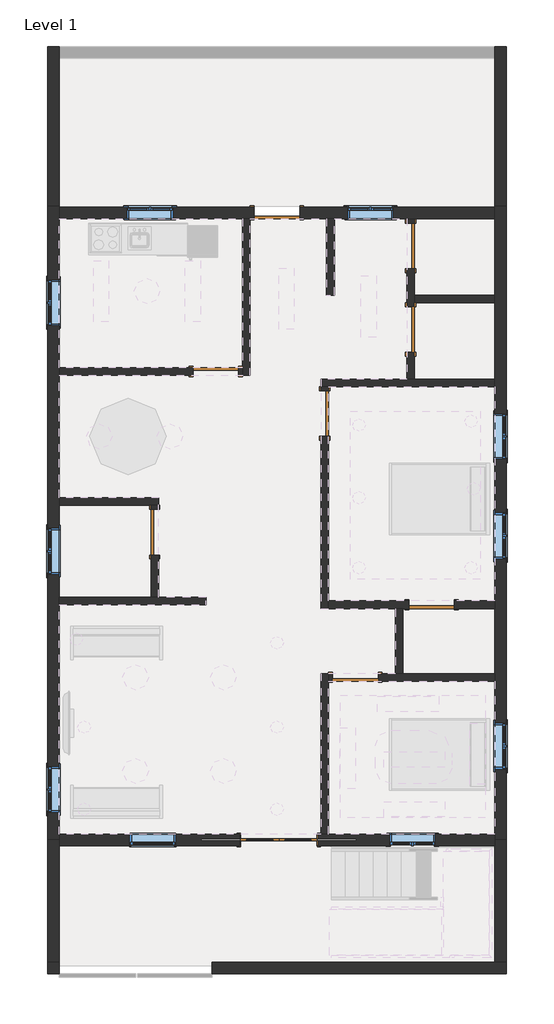
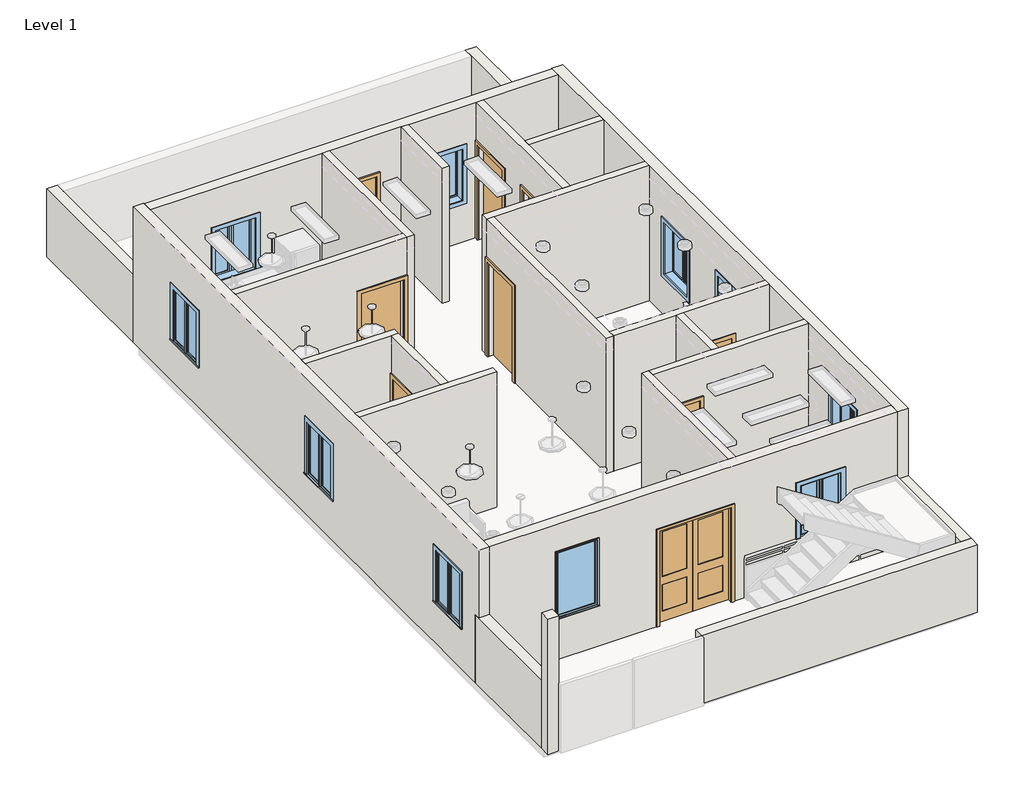
# One storey, part 1 of 2: 24 walls, 10 windows, 9 doors.
"""IFC4 building model written with IfcOpenShell, lengths in millimetres."""

from ifc_helpers import new_model, si_unit, frame, origin, origin_with_axes, place, context, project, spatial, polyline, outline, extrude, faceted_brep, transform, mapped, element, save
from components import door_53d589bd, door_0ca8825f, door_16372e1c, single_flush_single_door_686f89d2, window_419b5846, m_awning_with_trim_0915_x_1220mm_6739fb62

model = new_model("IFC4")

# Units and contexts
model_context = context("Model", 3, world=origin())
ifc_project = project(units=[si_unit("LENGTHUNIT", "METRE", prefix="MILLI")], contexts=[model_context])

# Site, building, storey
site = spatial("IfcSite", under=ifc_project)
building = spatial("IfcBuilding", under=site)
storey = spatial("IfcBuildingStorey", under=building, Name="Level 1", Elevation=0.0)

# Doors
placement = place(None, origin())
door_shape = door_53d589bd(model_context)
element("IfcDoor", 1, ObjectType="Door-Interior-Double-Pocket-2_Panel-Wood : 60\" x 84\"", at=placement, inside=storey, context=model_context, shape_type="MappedRepresentation", body=[
    mapped(door_shape, transform((-5459.0692849, 1586.5206867, 0.0), x_axis=(1.0, 0.0, 0.0), y_axis=(0.0, 1.0, 0.0), z_axis=(0.0, 0.0, 1.0))),
])
door_2_shape = door_0ca8825f(model_context)
element("IfcDoor", 2, ObjectType="Single-Flush : 36\" x 84\"", at=placement, inside=storey, context=model_context, shape_type="MappedRepresentation", body=[
    mapped(door_2_shape, transform((-5497.1692849, 14083.3206867, 0.0), x_axis=(-1.0, 0.0, 0.0), y_axis=(0.0, -1.0, 0.0), z_axis=(0.0, 0.0, 1.0))),
])
door_3_shape = door_16372e1c(model_context)
element("IfcDoor", 3, ObjectType="Single-Flush : 36\" x 84\"", at=placement, inside=storey, context=model_context, shape_type="MappedRepresentation", body=[
    mapped(door_3_shape, transform((-6716.3692849, 10921.0206867, 0.0), x_axis=(1.0, 0.0, 0.0), y_axis=(0.0, 1.0, 0.0), z_axis=(0.0, 0.0, 1.0))),
])
element("IfcDoor", 4, ObjectType="Single-Flush : single door", at=placement, inside=storey, context=model_context, shape_type="MappedRepresentation", body=[
    mapped(door_3_shape, transform((-3935.0692849, 4825.0206867, 0.0), x_axis=(-1.0, 0.0, 0.0), y_axis=(0.0, -1.0, 0.0), z_axis=(0.0, 0.0, 1.0))),
])
element("IfcDoor", 5, ObjectType="Single-Flush : single door", at=placement, inside=storey, context=model_context, shape_type="MappedRepresentation", body=[
    mapped(door_3_shape, transform((-2411.0692849, 6272.8206867, 0.0), x_axis=(-1.0, 0.0, 0.0), y_axis=(0.0, -1.0, 0.0), z_axis=(0.0, 0.0, 1.0))),
])
element("IfcDoor", 6, ObjectType="Single-Flush : single door", at=placement, inside=storey, context=model_context, shape_type="MappedRepresentation", body=[
    mapped(door_3_shape, transform((-7935.5692849, 7720.6206867, 0.0), x_axis=(0.0, 1.0, 0.0), y_axis=(-1.0, 0.0, 0.0), z_axis=(0.0, 0.0, 1.0))),
])
single_flush_single_door_shape = single_flush_single_door_686f89d2(model_context)
element("IfcDoor", 7, ObjectType="Single-Flush : single door", at=placement, inside=storey, context=model_context, shape_type="MappedRepresentation", body=[
    mapped(single_flush_single_door_shape, transform((-4544.6692849, 10082.8206867, 0.0), x_axis=(0.0, 1.0, 0.0), y_axis=(-1.0, 0.0, 0.0), z_axis=(0.0, 0.0, 1.0))),
])
element("IfcDoor", 8, ObjectType="Single-Flush : single door", at=placement, inside=storey, context=model_context, shape_type="MappedRepresentation", body=[
    mapped(single_flush_single_door_shape, transform((-2830.1692849, 13422.9206867, 0.0), x_axis=(0.0, 1.0, 0.0), y_axis=(-1.0, 0.0, 0.0), z_axis=(0.0, 0.0, 1.0))),
])
element("IfcDoor", 9, ObjectType="Single-Flush : single door", at=placement, inside=storey, context=model_context, shape_type="MappedRepresentation", body=[
    mapped(single_flush_single_door_shape, transform((-2830.1692849, 11759.2206867, 0.0), x_axis=(0.0, 1.0, 0.0), y_axis=(-1.0, 0.0, 0.0), z_axis=(0.0, 0.0, 1.0))),
])

# Walls
element("IfcWall", 10, ObjectType="6\"", at=placement, inside=storey, context=model_context, shape_type="Brep", body=[
    faceted_brep([(-4468.4692849, 1700.8206867, 0.0), (-4468.4692849, 4748.8206867, 0.0), (-4468.4692849, 4901.2206867, 0.0), (-4468.4692849, 4901.2206867, 3048.0), (-4468.4692849, 4748.8206867, 3048.0), (-4468.4692849, 1700.8206867, 3048.0), (-4620.8692849, 1700.8206867, 0.0), (-4620.8692849, 1700.8206867, 3048.0), (-4620.8692849, 4901.2206867, 3048.0), (-4620.8692849, 4901.2206867, 0.0)], [[[0, 1, 2, 3, 4, 5]], [[6, 7, 8, 9]], [[2, 1, 0, 6, 9]], [[5, 4, 3, 8, 7]], [[0, 5, 7, 6]], [[3, 2, 9, 8]]]),
])
element("IfcWall", 11, ObjectType="6\"", at=placement, inside=storey, context=model_context, shape_type="Brep", body=[
    faceted_brep([(-4392.2692849, 4901.2206867, 2133.6), (-4392.2692849, 4901.2206867, 0.0), (-4468.4692849, 4901.2206867, 0.0), (-4468.4692849, 4901.2206867, 3048.0), (-3134.9692849, 4901.2206867, 3048.0), (-2982.5692849, 4901.2206867, 3048.0), (-1153.7692849, 4901.2206867, 3048.0), (-1153.7692849, 4901.2206867, 0.0), (-2982.5692849, 4901.2206867, 0.0), (-3134.9692849, 4901.2206867, 0.0), (-3477.8692849, 4901.2206867, 0.0), (-3477.8692849, 4901.2206867, 2133.6), (-4468.4692849, 4748.8206867, 0.0), (-4392.2692849, 4748.8206867, 0.0), (-4392.2692849, 4748.8206867, 2133.6), (-3477.8692849, 4748.8206867, 2133.6), (-3477.8692849, 4748.8206867, 0.0), (-1153.7692849, 4748.8206867, 0.0), (-1153.7692849, 4748.8206867, 3048.0), (-4468.4692849, 4748.8206867, 3048.0)], [[[0, 1, 2, 3, 4, 5, 6, 7, 8, 9, 10, 11]], [[12, 13, 14, 15, 16, 17, 18, 19]], [[2, 1, 13, 12]], [[10, 9, 8, 7, 17, 16]], [[6, 5, 4, 3, 19, 18]], [[7, 6, 18, 17]], [[3, 2, 12, 19]], [[14, 13, 1, 0]], [[15, 14, 0, 11]], [[16, 15, 11, 10]]]),
])
element("IfcWall", 12, ObjectType="6\"", at=placement, inside=storey, context=model_context, shape_type="SweptSolid", body=[
    extrude(outline(polyline([(-2982.5692849, 6196.6206867), (-2982.5692849, 4901.2206867), (-3134.9692849, 4901.2206867), (-3134.9692849, 6196.6206867), (-2982.5692849, 6196.6206867)])), origin_with_axes(), (0.0, 0.0, 1.0), 3048.0),
])
element("IfcWall", 13, ObjectType="6\"", at=placement, inside=storey, context=model_context, shape_type="Brep", body=[
    faceted_brep([(-4468.4692849, 6349.0206867, 3048.0), (-1153.7692849, 6349.0206867, 3048.0), (-1153.7692849, 6349.0206867, 0.0), (-1953.8692849, 6349.0206867, 0.0), (-1953.8692849, 6349.0206867, 2133.6), (-2868.2692849, 6349.0206867, 2133.6), (-2868.2692849, 6349.0206867, 0.0), (-4468.4692849, 6349.0206867, 0.0), (-1153.7692849, 6196.6206867, 3048.0), (-2982.5692849, 6196.6206867, 3048.0), (-3134.9692849, 6196.6206867, 3048.0), (-4468.4692849, 6196.6206867, 3048.0), (-4468.4692849, 6196.6206867, 0.0), (-3134.9692849, 6196.6206867, 0.0), (-2982.5692849, 6196.6206867, 0.0), (-2868.2692849, 6196.6206867, 0.0), (-2868.2692849, 6196.6206867, 2133.6), (-1953.8692849, 6196.6206867, 2133.6), (-1953.8692849, 6196.6206867, 0.0), (-1153.7692849, 6196.6206867, 0.0)], [[[0, 1, 2, 3, 4, 5, 6, 7]], [[8, 9, 10, 11, 12, 13, 14, 15, 16, 17, 18, 19]], [[2, 19, 18, 3]], [[12, 7, 6, 15, 14, 13]], [[1, 0, 11, 10, 9, 8]], [[2, 1, 8, 19]], [[0, 7, 12, 11]], [[16, 5, 4, 17]], [[17, 4, 3, 18]], [[5, 16, 15, 6]]]),
])
element("IfcWall", 14, ObjectType="6\"", at=placement, inside=storey, context=model_context, shape_type="Brep", body=[
    faceted_brep([(-1153.7692849, 10768.6206867, 0.0), (-2753.9692849, 10768.6206867, 0.0), (-2906.3692849, 10768.6206867, 0.0), (-4620.8692849, 10768.6206867, 0.0), (-4620.8692849, 10768.6206867, 3048.0), (-2906.3692849, 10768.6206867, 3048.0), (-2753.9692849, 10768.6206867, 3048.0), (-1153.7692849, 10768.6206867, 3048.0), (-1153.7692849, 10616.2206867, 0.0), (-1153.7692849, 10616.2206867, 3048.0), (-4468.4692849, 10616.2206867, 3048.0), (-4620.8692849, 10616.2206867, 3048.0), (-4620.8692849, 10616.2206867, 0.0), (-4468.4692849, 10616.2206867, 0.0)], [[[0, 1, 2, 3, 4, 5, 6, 7]], [[8, 9, 10, 11, 12, 13]], [[3, 2, 1, 0, 8, 13, 12]], [[7, 6, 5, 4, 11, 10, 9]], [[0, 7, 9, 8]], [[4, 3, 12, 11]]]),
])
element("IfcWall", 15, ObjectType="6\"", at=placement, inside=storey, context=model_context, shape_type="Brep", body=[
    faceted_brep([(-4468.4692849, 10540.0206867, 2133.6), (-4468.4692849, 10540.0206867, 0.0), (-4468.4692849, 10616.2206867, 0.0), (-4468.4692849, 10616.2206867, 3048.0), (-4468.4692849, 6349.0206867, 3048.0), (-4468.4692849, 6196.6206867, 3048.0), (-4468.4692849, 6196.6206867, 0.0), (-4468.4692849, 6349.0206867, 0.0), (-4468.4692849, 9625.6206867, 0.0), (-4468.4692849, 9625.6206867, 2133.6), (-4620.8692849, 10616.2206867, 0.0), (-4620.8692849, 10540.0206867, 0.0), (-4620.8692849, 10540.0206867, 2133.6), (-4620.8692849, 9625.6206867, 2133.6), (-4620.8692849, 9625.6206867, 0.0), (-4620.8692849, 6196.6206867, 0.0), (-4620.8692849, 6196.6206867, 3048.0), (-4620.8692849, 10616.2206867, 3048.0)], [[[0, 1, 2, 3, 4, 5, 6, 7, 8, 9]], [[10, 11, 12, 13, 14, 15, 16, 17]], [[2, 1, 11, 10]], [[8, 7, 6, 15, 14]], [[5, 4, 3, 17, 16]], [[3, 2, 10, 17]], [[6, 5, 16, 15]], [[12, 11, 1, 0]], [[13, 12, 0, 9]], [[14, 13, 9, 8]]]),
])
element("IfcWall", 16, ObjectType="6\"", at=placement, inside=storey, context=model_context, shape_type="SweptSolid", body=[
    extrude(outline(polyline([(-2753.9692849, 12445.0206867), (-1153.7692849, 12445.0206867), (-1153.7692849, 12292.6206867), (-2753.9692849, 12292.6206867), (-2753.9692849, 12445.0206867)])), origin_with_axes(), (0.0, 0.0, 1.0), 3048.0),
])
element("IfcWall", 17, ObjectType="6\"", at=placement, inside=storey, context=model_context, shape_type="Brep", body=[
    faceted_brep([(-2753.9692849, 12216.4206867, 2133.6), (-2753.9692849, 12216.4206867, 0.0), (-2753.9692849, 12292.6206867, 0.0), (-2753.9692849, 12445.0206867, 0.0), (-2753.9692849, 12965.7206867, 0.0), (-2753.9692849, 12965.7206867, 2133.6), (-2753.9692849, 13880.1206867, 2133.6), (-2753.9692849, 13880.1206867, 0.0), (-2753.9692849, 13969.0206867, 0.0), (-2753.9692849, 13969.0206867, 3048.0), (-2753.9692849, 12445.0206867, 3048.0), (-2753.9692849, 12292.6206867, 3048.0), (-2753.9692849, 10768.6206867, 3048.0), (-2753.9692849, 10768.6206867, 0.0), (-2753.9692849, 11302.0206867, 0.0), (-2753.9692849, 11302.0206867, 2133.6), (-2906.3692849, 12965.7206867, 0.0), (-2906.3692849, 12216.4206867, 0.0), (-2906.3692849, 12216.4206867, 2133.6), (-2906.3692849, 11302.0206867, 2133.6), (-2906.3692849, 11302.0206867, 0.0), (-2906.3692849, 10768.6206867, 0.0), (-2906.3692849, 10768.6206867, 3048.0), (-2906.3692849, 13969.0206867, 3048.0), (-2906.3692849, 13969.0206867, 0.0), (-2906.3692849, 13880.1206867, 0.0), (-2906.3692849, 13880.1206867, 2133.6), (-2906.3692849, 12965.7206867, 2133.6)], [[[0, 1, 2, 3, 4, 5, 6, 7, 8, 9, 10, 11, 12, 13, 14, 15]], [[16, 17, 18, 19, 20, 21, 22, 23, 24, 25, 26, 27]], [[8, 7, 25, 24]], [[14, 13, 21, 20]], [[4, 3, 2, 1, 17, 16]], [[12, 11, 10, 9, 23, 22]], [[13, 12, 22, 21]], [[9, 8, 24, 23]], [[26, 25, 7, 6]], [[27, 26, 6, 5]], [[16, 27, 5, 4]], [[18, 17, 1, 0]], [[19, 18, 0, 15]], [[20, 19, 15, 14]]]),
])
element("IfcWall", 18, ObjectType="6\"", at=placement, inside=storey, context=model_context, shape_type="Brep", body=[
    faceted_brep([(-6182.9692849, 13969.0206867, 0.0), (-6182.9692849, 10997.2206867, 0.0), (-6182.9692849, 10844.8206867, 0.0), (-6182.9692849, 10844.8206867, 3048.0), (-6182.9692849, 10997.2206867, 3048.0), (-6182.9692849, 13969.0206867, 3048.0), (-6030.5692849, 13969.0206867, 0.0), (-6030.5692849, 13969.0206867, 3048.0), (-6030.5692849, 10844.8206867, 3048.0), (-6030.5692849, 10844.8206867, 0.0)], [[[0, 1, 2, 3, 4, 5]], [[6, 7, 8, 9]], [[2, 1, 0, 6, 9]], [[5, 4, 3, 8, 7]], [[0, 5, 7, 6]], [[3, 2, 9, 8]]]),
])
element("IfcWall", 19, ObjectType="6\"", at=placement, inside=storey, context=model_context, shape_type="Brep", body=[
    faceted_brep([(-9840.5692849, 8254.0206867, 0.0), (-8011.7692849, 8254.0206867, 0.0), (-7859.3692849, 8254.0206867, 0.0), (-7859.3692849, 8254.0206867, 3048.0), (-8011.7692849, 8254.0206867, 3048.0), (-9840.5692849, 8254.0206867, 3048.0), (-9840.5692849, 8406.4206867, 0.0), (-9840.5692849, 8406.4206867, 3048.0), (-7859.3692849, 8406.4206867, 3048.0), (-7859.3692849, 8406.4206867, 0.0)], [[[0, 1, 2, 3, 4, 5]], [[6, 7, 8, 9]], [[2, 1, 0, 6, 9]], [[5, 4, 3, 8, 7]], [[0, 5, 7, 6]], [[3, 2, 9, 8]]]),
])
element("IfcWall", 20, ObjectType="6\"", at=placement, inside=storey, context=model_context, shape_type="SweptSolid", body=[
    extrude(outline(polyline([(8254.0206867, 0.0), (8177.8206867, 0.0), (8177.8206867, 2133.6), (7263.4206867, 2133.6), (7263.4206867, 0.0), (6425.2206867, 0.0), (6425.2206867, 3048.0), (8254.0206867, 3048.0), (8254.0206867, 0.0)])), frame((-8011.7692849, 0.0, 0.0), z_axis=(1.0, 0.0, 0.0), x_axis=(0.0, 1.0, 0.0)), (0.0, 0.0, 1.0), 152.4),
])
element("IfcWall", 21, ObjectType="6\"", at=placement, inside=storey, context=model_context, shape_type="Brep", body=[
    faceted_brep([(-6906.8692849, 6425.2206867, 0.0), (-7859.3692849, 6425.2206867, 0.0), (-8011.7692849, 6425.2206867, 0.0), (-9840.5692849, 6425.2206867, 0.0), (-9840.5692849, 6425.2206867, 3048.0), (-8011.7692849, 6425.2206867, 3048.0), (-7859.3692849, 6425.2206867, 3048.0), (-6906.8692849, 6425.2206867, 3048.0), (-6906.8692849, 6272.8206867, 0.0), (-6906.8692849, 6272.8206867, 3048.0), (-9840.5692849, 6272.8206867, 3048.0), (-9840.5692849, 6272.8206867, 0.0)], [[[0, 1, 2, 3, 4, 5, 6, 7]], [[8, 9, 10, 11]], [[3, 2, 1, 0, 8, 11]], [[7, 6, 5, 4, 10, 9]], [[0, 7, 9, 8]], [[4, 3, 11, 10]]]),
])
element("IfcWall", 22, ObjectType="6\"", at=placement, inside=storey, context=model_context, shape_type="SweptSolid", body=[
    extrude(outline(polyline([(2133.6, -6259.1692849), (0.0, -6259.1692849), (0.0, -6182.9692849), (3048.0, -6182.9692849), (3048.0, -9840.5692849), (0.0, -9840.5692849), (0.0, -7173.5692849), (2133.6, -7173.5692849), (2133.6, -6259.1692849)])), frame((0.0, 10844.8206867, 0.0), z_axis=(0.0, 1.0, 0.0), x_axis=(0.0, 0.0, 1.0)), (0.0, 0.0, 1.0), 152.4),
])
element("IfcWall", 23, ObjectType="6\"", at=placement, inside=storey, context=model_context, shape_type="SweptSolid", body=[
    extrude(outline(polyline([(-4506.5692849, 12445.0206867), (-4506.5692849, 13969.0206867), (-4354.1692849, 13969.0206867), (-4354.1692849, 12445.0206867), (-4506.5692849, 12445.0206867)])), origin_with_axes(), (0.0, 0.0, 1.0), 3048.0),
])
element("IfcWall", 24, ObjectType="9\"", at=placement, inside=storey, context=model_context, shape_type="Brep", body=[
    faceted_brep([(-9840.5692849, -851.8793133, 0.0), (-9840.5692849, 1472.2206867, 0.0), (-9840.5692849, 1586.5206867, 0.0), (-9840.5692849, 1586.5206867, 1524.0), (-9840.5692849, 1472.2206867, 1524.0), (-9840.5692849, -851.8793133, 1524.0), (-10069.1692849, -851.8793133, 0.0), (-10069.1692849, -851.8793133, 1524.0), (-10069.1692849, 1472.2206867, 1524.0), (-10069.1692849, 1586.5206867, 1524.0), (-10069.1692849, 1586.5206867, 0.0)], [[[0, 1, 2, 3, 4, 5]], [[6, 7, 8, 9, 10]], [[2, 1, 0, 6, 10]], [[3, 2, 10, 9]], [[5, 4, 3, 9, 8, 7]], [[0, 5, 7, 6]]]),
])
element("IfcWall", 25, ObjectType="9\"", at=placement, inside=storey, context=model_context, shape_type="Brep", body=[
    faceted_brep([(-1153.7692849, 17398.0206867, 0.0), (-1153.7692849, 17169.4206867, 0.0), (-1153.7692849, 14210.3206867, 0.0), (-1153.7692849, 14210.3206867, 1524.0), (-1153.7692849, 17169.4206867, 1524.0), (-1153.7692849, 17398.0206867, 1524.0), (-925.1692849, 17398.0206867, 0.0), (-925.1692849, 17398.0206867, 1524.0), (-925.1692849, 14210.3206867, 1524.0), (-925.1692849, 14210.3206867, 0.0)], [[[0, 1, 2, 3, 4, 5]], [[6, 7, 8, 9]], [[2, 1, 0, 6, 9]], [[3, 2, 9, 8]], [[5, 4, 3, 8, 7]], [[0, 5, 7, 6]]]),
])
element("IfcWall", 26, ObjectType="9\"", at=placement, inside=storey, context=model_context, shape_type="Brep", body=[
    faceted_brep([(-9840.5692849, 1700.8206867, 3048.0), (-4620.8692849, 1700.8206867, 3048.0), (-4468.4692849, 1700.8206867, 3048.0), (-1153.7692849, 1700.8206867, 3048.0), (-1153.7692849, 1700.8206867, 0.0), (-4468.4692849, 1700.8206867, 0.0), (-4620.8692849, 1700.8206867, 0.0), (-4671.6692849, 1700.8206867, 0.0), (-4671.6692849, 1700.8206867, 2159.0), (-6246.4692849, 1700.8206867, 2159.0), (-6246.4692849, 1700.8206867, 0.0), (-9840.5692849, 1700.8206867, 0.0), (-3249.2692849, 1700.8206867, 2133.6), (-3249.2692849, 1700.8206867, 914.4), (-2334.8692849, 1700.8206867, 914.4), (-2334.8692849, 1700.8206867, 2133.6), (-8431.1692849, 1700.8206867, 2439.0), (-8431.1692849, 1700.8206867, 915.0), (-7516.1692849, 1700.8206867, 915.0), (-7516.1692849, 1700.8206867, 2439.0), (-1153.7692849, 1472.2206867, 3048.0), (-9840.5692849, 1472.2206867, 3048.0), (-9840.5692849, 1472.2206867, 1524.0), (-9840.5692849, 1472.2206867, 0.0), (-6246.4692849, 1472.2206867, 0.0), (-6246.4692849, 1472.2206867, 2159.0), (-4671.6692849, 1472.2206867, 2159.0), (-4671.6692849, 1472.2206867, 0.0), (-1153.7692849, 1472.2206867, 0.0), (-1153.7692849, 1472.2206867, 1524.0), (-3249.2692849, 1472.2206867, 2133.6), (-2334.8692849, 1472.2206867, 2133.6), (-2334.8692849, 1472.2206867, 914.4), (-3249.2692849, 1472.2206867, 914.4), (-8431.1692849, 1472.2206867, 2439.0), (-7516.1692849, 1472.2206867, 2439.0), (-7516.1692849, 1472.2206867, 915.0), (-8431.1692849, 1472.2206867, 915.0), (-1153.7692849, 1586.5206867, 0.0), (-4671.6692849, 1565.8831867, 0.0), (-3909.6692849, 1565.8831867, 0.0), (-3909.6692849, 1607.1581867, 0.0), (-4671.6692849, 1607.1581867, 0.0), (-9840.5692849, 1586.5206867, 0.0), (-6246.4692849, 1607.1581867, 0.0), (-7008.4692849, 1607.1581867, 0.0), (-7008.4692849, 1565.8831867, 0.0), (-6246.4692849, 1565.8831867, 0.0), (-3909.6692849, 1607.1581867, 2159.0), (-3909.6692849, 1565.8831867, 2159.0), (-4671.6692849, 1565.8831867, 2159.0), (-6246.4692849, 1565.8831867, 2159.0), (-7008.4692849, 1565.8831867, 2159.0), (-7008.4692849, 1607.1581867, 2159.0), (-6246.4692849, 1607.1581867, 2159.0), (-4671.6692849, 1607.1581867, 2159.0)], [[[0, 1, 2, 3, 4, 5, 6, 7, 8, 9, 10, 11], [12, 13, 14, 15], [16, 17, 18, 19]], [[20, 21, 22, 23, 24, 25, 26, 27, 28, 29], [30, 31, 32, 33], [34, 35, 36, 37]], [[4, 38, 28, 27, 39, 40, 41, 42, 7, 6, 5]], [[23, 43, 11, 10, 44, 45, 46, 47, 24]], [[3, 2, 1, 0, 21, 20]], [[13, 12, 30, 33]], [[14, 13, 33, 32]], [[15, 14, 32, 31]], [[12, 15, 31, 30]], [[48, 49, 50, 26, 25, 51, 52, 53, 54, 9, 8, 55]], [[48, 55, 42, 41]], [[55, 8, 7, 42]], [[9, 54, 44, 10]], [[54, 53, 45, 44]], [[53, 52, 46, 45]], [[52, 51, 47, 46]], [[51, 25, 24, 47]], [[26, 50, 39, 27]], [[50, 49, 40, 39]], [[49, 48, 41, 40]], [[11, 43, 23, 22, 21, 0]], [[28, 38, 4, 3, 20, 29]], [[17, 16, 34, 37]], [[18, 17, 37, 36]], [[19, 18, 36, 35]], [[16, 19, 35, 34]]]),
])
element("IfcWall", 27, ObjectType="9\"", at=placement, inside=storey, context=model_context, shape_type="Brep", body=[
    faceted_brep([(-5954.3692849, 14197.6206867, 2133.6), (-5954.3692849, 14197.6206867, 0.0), (-9840.5692849, 14197.6206867, 0.0), (-9840.5692849, 14197.6206867, 3048.0), (-1153.7692849, 14197.6206867, 3048.0), (-1153.7692849, 14197.6206867, 0.0), (-5039.9692849, 14197.6206867, 0.0), (-5039.9692849, 14197.6206867, 2133.6), (-7573.6192849, 14197.6206867, 2133.6), (-8488.0192849, 14197.6206867, 2133.6), (-8488.0192849, 14197.6206867, 914.4), (-7573.6192849, 14197.6206867, 914.4), (-3173.0692849, 14197.6206867, 2133.6), (-4087.4692849, 14197.6206867, 2133.6), (-4087.4692849, 14197.6206867, 914.4), (-3173.0692849, 14197.6206867, 914.4), (-9840.5692849, 13969.0206867, 0.0), (-6182.9692849, 13969.0206867, 0.0), (-6030.5692849, 13969.0206867, 0.0), (-5954.3692849, 13969.0206867, 0.0), (-5954.3692849, 13969.0206867, 2133.6), (-5039.9692849, 13969.0206867, 2133.6), (-5039.9692849, 13969.0206867, 0.0), (-4506.5692849, 13969.0206867, 0.0), (-4354.1692849, 13969.0206867, 0.0), (-2906.3692849, 13969.0206867, 0.0), (-2753.9692849, 13969.0206867, 0.0), (-1153.7692849, 13969.0206867, 0.0), (-1153.7692849, 13969.0206867, 3048.0), (-2753.9692849, 13969.0206867, 3048.0), (-2906.3692849, 13969.0206867, 3048.0), (-4354.1692849, 13969.0206867, 3048.0), (-4506.5692849, 13969.0206867, 3048.0), (-6030.5692849, 13969.0206867, 3048.0), (-6182.9692849, 13969.0206867, 3048.0), (-9840.5692849, 13969.0206867, 3048.0), (-7573.6192849, 13969.0206867, 2133.6), (-7573.6192849, 13969.0206867, 914.4), (-8488.0192849, 13969.0206867, 914.4), (-8488.0192849, 13969.0206867, 2133.6), (-3173.0692849, 13969.0206867, 2133.6), (-3173.0692849, 13969.0206867, 914.4), (-4087.4692849, 13969.0206867, 914.4), (-4087.4692849, 13969.0206867, 2133.6)], [[[0, 1, 2, 3, 4, 5, 6, 7], [8, 9, 10, 11], [12, 13, 14, 15]], [[16, 17, 18, 19, 20, 21, 22, 23, 24, 25, 26, 27, 28, 29, 30, 31, 32, 33, 34, 35], [36, 37, 38, 39], [40, 41, 42, 43]], [[6, 5, 27, 26, 25, 24, 23, 22]], [[2, 1, 19, 18, 17, 16]], [[4, 3, 35, 34, 33, 32, 31, 30, 29, 28]], [[3, 2, 16, 35]], [[5, 4, 28, 27]], [[37, 36, 8, 11]], [[38, 37, 11, 10]], [[39, 38, 10, 9]], [[36, 39, 9, 8]], [[41, 40, 12, 15]], [[42, 41, 15, 14]], [[43, 42, 14, 13]], [[40, 43, 13, 12]], [[20, 19, 1, 0]], [[21, 20, 0, 7]], [[22, 21, 7, 6]]]),
])
element("IfcWall", 28, ObjectType="9\"", at=placement, inside=storey, context=model_context, shape_type="Brep", body=[
    faceted_brep([(-9840.5692849, 1586.5206867, 0.0), (-9840.5692849, 1700.8206867, 0.0), (-9840.5692849, 6272.8206867, 0.0), (-9840.5692849, 6425.2206867, 0.0), (-9840.5692849, 8254.0206867, 0.0), (-9840.5692849, 8406.4206867, 0.0), (-9840.5692849, 10844.8206867, 0.0), (-9840.5692849, 10997.2206867, 0.0), (-9840.5692849, 13969.0206867, 0.0), (-9840.5692849, 14197.6206867, 0.0), (-9840.5692849, 14210.3206867, 0.0), (-9840.5692849, 14210.3206867, 1524.0), (-9840.5692849, 14210.3206867, 3048.0), (-9840.5692849, 14197.6206867, 3048.0), (-9840.5692849, 13969.0206867, 3048.0), (-9840.5692849, 10997.2206867, 3048.0), (-9840.5692849, 10844.8206867, 3048.0), (-9840.5692849, 8406.4206867, 3048.0), (-9840.5692849, 8254.0206867, 3048.0), (-9840.5692849, 6425.2206867, 3048.0), (-9840.5692849, 6272.8206867, 3048.0), (-9840.5692849, 1700.8206867, 3048.0), (-9840.5692849, 1472.2206867, 3048.0), (-9840.5692849, 1472.2206867, 1524.0), (-9840.5692849, 1586.5206867, 1524.0), (-9840.5692849, 3047.0206867, 2133.6), (-9840.5692849, 3047.0206867, 914.4), (-9840.5692849, 2132.6206867, 914.4), (-9840.5692849, 2132.6206867, 2133.6), (-9840.5692849, 7796.8206867, 2133.6), (-9840.5692849, 7796.8206867, 914.4), (-9840.5692849, 6882.4206867, 914.4), (-9840.5692849, 6882.4206867, 2133.6), (-9840.5692849, 12749.8206867, 2133.6), (-9840.5692849, 12749.8206867, 914.4), (-9840.5692849, 11835.4206867, 914.4), (-9840.5692849, 11835.4206867, 2133.6), (-10069.1692849, 1586.5206867, 0.0), (-10069.1692849, 1586.5206867, 1524.0), (-10069.1692849, 1472.2206867, 1524.0), (-10069.1692849, 1472.2206867, 3048.0), (-10069.1692849, 14210.3206867, 3048.0), (-10069.1692849, 14210.3206867, 1524.0), (-10069.1692849, 14210.3206867, 0.0), (-10069.1692849, 3047.0206867, 2133.6), (-10069.1692849, 2132.6206867, 2133.6), (-10069.1692849, 2132.6206867, 914.4), (-10069.1692849, 3047.0206867, 914.4), (-10069.1692849, 7796.8206867, 2133.6), (-10069.1692849, 6882.4206867, 2133.6), (-10069.1692849, 6882.4206867, 914.4), (-10069.1692849, 7796.8206867, 914.4), (-10069.1692849, 12749.8206867, 2133.6), (-10069.1692849, 11835.4206867, 2133.6), (-10069.1692849, 11835.4206867, 914.4), (-10069.1692849, 12749.8206867, 914.4)], [[[0, 1, 2, 3, 4, 5, 6, 7, 8, 9, 10, 11, 12, 13, 14, 15, 16, 17, 18, 19, 20, 21, 22, 23, 24], [25, 26, 27, 28], [29, 30, 31, 32], [33, 34, 35, 36]], [[37, 38, 39, 40, 41, 42, 43], [44, 45, 46, 47], [48, 49, 50, 51], [52, 53, 54, 55]], [[10, 9, 8, 7, 6, 5, 4, 3, 2, 1, 0, 37, 43]], [[12, 11, 10, 43, 42, 41]], [[22, 21, 20, 19, 18, 17, 16, 15, 14, 13, 12, 41, 40]], [[25, 28, 45, 44]], [[28, 27, 46, 45]], [[27, 26, 47, 46]], [[26, 25, 44, 47]], [[29, 32, 49, 48]], [[32, 31, 50, 49]], [[31, 30, 51, 50]], [[30, 29, 48, 51]], [[33, 36, 53, 52]], [[36, 35, 54, 53]], [[35, 34, 55, 54]], [[34, 33, 52, 55]], [[0, 24, 38, 37]], [[23, 39, 38, 24]], [[23, 22, 40, 39]]]),
])
element("IfcWall", 29, ObjectType="9\"", at=placement, inside=storey, context=model_context, shape_type="Brep", body=[
    faceted_brep([(-1153.7692849, 1586.5206867, 0.0), (-1153.7692849, 1472.2206867, 0.0), (-1153.7692849, -851.8793133, 0.0), (-1153.7692849, -851.8793133, 1524.0), (-1153.7692849, 1472.2206867, 1524.0), (-1153.7692849, 1586.5206867, 1524.0), (-925.1692849, 1586.5206867, 0.0), (-925.1692849, 1586.5206867, 1524.0), (-925.1692849, 1472.2206867, 1524.0), (-925.1692849, -851.8793133, 1524.0), (-925.1692849, -851.8793133, 0.0)], [[[0, 1, 2, 3, 4, 5]], [[6, 7, 8, 9, 10]], [[2, 1, 0, 6, 10]], [[5, 4, 3, 9, 8, 7]], [[0, 5, 7, 6]], [[3, 2, 10, 9]]]),
])
element("IfcWall", 30, ObjectType="9\"", at=placement, inside=storey, context=model_context, shape_type="Brep", body=[
    faceted_brep([(-9840.5692849, 14210.3206867, 0.0), (-9840.5692849, 17169.4206867, 0.0), (-9840.5692849, 17398.0206867, 0.0), (-9840.5692849, 17398.0206867, 1524.0), (-9840.5692849, 17169.4206867, 1524.0), (-9840.5692849, 14210.3206867, 1524.0), (-10069.1692849, 14210.3206867, 0.0), (-10069.1692849, 14210.3206867, 1524.0), (-10069.1692849, 17398.0206867, 1524.0), (-10069.1692849, 17398.0206867, 0.0)], [[[0, 1, 2, 3, 4, 5]], [[6, 7, 8, 9]], [[2, 1, 0, 6, 9]], [[5, 4, 3, 8, 7]], [[0, 5, 7, 6]], [[3, 2, 9, 8]]]),
])
element("IfcWall", 31, ObjectType="9\"", at=placement, inside=storey, context=model_context, shape_type="Brep", body=[
    faceted_brep([(-1153.7692849, 14210.3206867, 0.0), (-1153.7692849, 14197.6206867, 0.0), (-1153.7692849, 13969.0206867, 0.0), (-1153.7692849, 12445.0206867, 0.0), (-1153.7692849, 12292.6206867, 0.0), (-1153.7692849, 10768.6206867, 0.0), (-1153.7692849, 10616.2206867, 0.0), (-1153.7692849, 6349.0206867, 0.0), (-1153.7692849, 6196.6206867, 0.0), (-1153.7692849, 4901.2206867, 0.0), (-1153.7692849, 4748.8206867, 0.0), (-1153.7692849, 1700.8206867, 0.0), (-1153.7692849, 1586.5206867, 0.0), (-1153.7692849, 1586.5206867, 1524.0), (-1153.7692849, 1472.2206867, 1524.0), (-1153.7692849, 1472.2206867, 3048.0), (-1153.7692849, 1700.8206867, 3048.0), (-1153.7692849, 4748.8206867, 3048.0), (-1153.7692849, 4901.2206867, 3048.0), (-1153.7692849, 6196.6206867, 3048.0), (-1153.7692849, 6349.0206867, 3048.0), (-1153.7692849, 10616.2206867, 3048.0), (-1153.7692849, 10768.6206867, 3048.0), (-1153.7692849, 12292.6206867, 3048.0), (-1153.7692849, 12445.0206867, 3048.0), (-1153.7692849, 13969.0206867, 3048.0), (-1153.7692849, 14197.6206867, 3048.0), (-1153.7692849, 14210.3206867, 3048.0), (-1153.7692849, 14210.3206867, 1524.0), (-1153.7692849, 9168.4206867, 2133.6), (-1153.7692849, 9168.4206867, 914.4), (-1153.7692849, 10082.8206867, 914.4), (-1153.7692849, 10082.8206867, 2133.6), (-1153.7692849, 7187.2206867, 2133.6), (-1153.7692849, 7187.2206867, 914.4), (-1153.7692849, 8101.6206867, 914.4), (-1153.7692849, 8101.6206867, 2133.6), (-1153.7692849, 2996.2206867, 2133.6), (-1153.7692849, 2996.2206867, 914.4), (-1153.7692849, 3910.6206867, 914.4), (-1153.7692849, 3910.6206867, 2133.6), (-925.1692849, 14210.3206867, 0.0), (-925.1692849, 14210.3206867, 1524.0), (-925.1692849, 14210.3206867, 3048.0), (-925.1692849, 1472.2206867, 3048.0), (-925.1692849, 1472.2206867, 1524.0), (-925.1692849, 1586.5206867, 1524.0), (-925.1692849, 1586.5206867, 0.0), (-925.1692849, 9168.4206867, 2133.6), (-925.1692849, 10082.8206867, 2133.6), (-925.1692849, 10082.8206867, 914.4), (-925.1692849, 9168.4206867, 914.4), (-925.1692849, 7187.2206867, 2133.6), (-925.1692849, 8101.6206867, 2133.6), (-925.1692849, 8101.6206867, 914.4), (-925.1692849, 7187.2206867, 914.4), (-925.1692849, 2996.2206867, 2133.6), (-925.1692849, 3910.6206867, 2133.6), (-925.1692849, 3910.6206867, 914.4), (-925.1692849, 2996.2206867, 914.4)], [[[0, 1, 2, 3, 4, 5, 6, 7, 8, 9, 10, 11, 12, 13, 14, 15, 16, 17, 18, 19, 20, 21, 22, 23, 24, 25, 26, 27, 28], [29, 30, 31, 32], [33, 34, 35, 36], [37, 38, 39, 40]], [[41, 42, 43, 44, 45, 46, 47], [48, 49, 50, 51], [52, 53, 54, 55], [56, 57, 58, 59]], [[12, 11, 10, 9, 8, 7, 6, 5, 4, 3, 2, 1, 0, 41, 47]], [[27, 26, 25, 24, 23, 22, 21, 20, 19, 18, 17, 16, 15, 44, 43]], [[0, 28, 27, 43, 42, 41]], [[29, 32, 49, 48]], [[32, 31, 50, 49]], [[31, 30, 51, 50]], [[30, 29, 48, 51]], [[33, 36, 53, 52]], [[36, 35, 54, 53]], [[35, 34, 55, 54]], [[34, 33, 52, 55]], [[37, 40, 57, 56]], [[40, 39, 58, 57]], [[39, 38, 59, 58]], [[38, 37, 56, 59]], [[13, 12, 47, 46]], [[45, 14, 13, 46]], [[15, 14, 45, 44]]]),
])
element("IfcWall", 32, ObjectType="9\"", at=placement, inside=storey, context=model_context, shape_type="Brep", body=[
    faceted_brep([(-10069.1692849, -1080.4793133, 0.0), (-9840.5692849, -1080.4793133, 0.0), (-9840.5692849, -1080.4793133, 3048.0), (-10069.1692849, -1080.4793133, 3048.0), (-10069.1692849, -851.8793133, 0.0), (-10069.1692849, -851.8793133, 1524.0), (-10069.1692849, -851.8793133, 3048.0), (-9840.5692849, -851.8793133, 3048.0), (-9840.5692849, -851.8793133, 1524.0), (-9840.5692849, -851.8793133, 0.0)], [[[0, 1, 2, 3]], [[4, 5, 6, 7, 8, 9]], [[1, 0, 4, 9]], [[2, 1, 9, 8, 7]], [[3, 2, 7, 6]], [[0, 3, 6, 5, 4]]]),
])
element("IfcWall", 33, ObjectType="9\"", at=placement, inside=storey, context=model_context, shape_type="Brep", body=[
    faceted_brep([(-6792.5692849, -1080.4793133, 0.0), (-925.1692849, -1080.4793133, 0.0), (-925.1692849, -1080.4793133, 1524.0), (-6792.5692849, -1080.4793133, 1524.0), (-6792.5692849, -851.8793133, 0.0), (-6792.5692849, -851.8793133, 1524.0), (-1153.7692849, -851.8793133, 1524.0), (-925.1692849, -851.8793133, 1524.0), (-925.1692849, -851.8793133, 0.0), (-1153.7692849, -851.8793133, 0.0)], [[[0, 1, 2, 3]], [[4, 5, 6, 7, 8, 9]], [[1, 0, 4, 9, 8]], [[3, 2, 7, 6, 5]], [[0, 3, 5, 4]], [[2, 1, 8, 7]]]),
])

# Windows
window_shape = window_419b5846(model_context)
element("IfcWindow", 34, ObjectType="Casement Dbl with Trim : 48\" x 48\"", at=placement, inside=storey, context=model_context, shape_type="MappedRepresentation", body=[
    mapped(window_shape, transform((-9935.8192849, 2589.8206867, 0.0), x_axis=(0.0, 1.0, 0.0), y_axis=(-1.0, 0.0, 0.0), z_axis=(0.0, 0.0, 1.0))),
])
element("IfcWindow", 35, ObjectType="Casement Dbl with Trim : 48\" x 48\"", at=placement, inside=storey, context=model_context, shape_type="MappedRepresentation", body=[
    mapped(window_shape, transform((-9935.8192849, 7339.6206867, 0.0), x_axis=(0.0, 1.0, 0.0), y_axis=(-1.0, 0.0, 0.0), z_axis=(0.0, 0.0, 1.0))),
])
element("IfcWindow", 36, ObjectType="Casement Dbl with Trim : 48\" x 48\"", at=placement, inside=storey, context=model_context, shape_type="MappedRepresentation", body=[
    mapped(window_shape, transform((-9935.8192849, 12292.6206867, 0.0), x_axis=(0.0, 1.0, 0.0), y_axis=(-1.0, 0.0, 0.0), z_axis=(0.0, 0.0, 1.0))),
])
element("IfcWindow", 37, ObjectType="Casement Dbl with Trim : 48\" x 48\"", at=placement, inside=storey, context=model_context, shape_type="MappedRepresentation", body=[
    mapped(window_shape, transform((-8030.8192849, 14064.2706867, 0.0), x_axis=(1.0, 0.0, 0.0), y_axis=(0.0, 1.0, 0.0), z_axis=(0.0, 0.0, 1.0))),
])
element("IfcWindow", 38, ObjectType="Casement Dbl with Trim : 48\" x 48\"", at=placement, inside=storey, context=model_context, shape_type="MappedRepresentation", body=[
    mapped(window_shape, transform((-3630.2692849, 14064.2706867, 0.0), x_axis=(1.0, 0.0, 0.0), y_axis=(0.0, 1.0, 0.0), z_axis=(0.0, 0.0, 1.0))),
])
element("IfcWindow", 39, ObjectType="Casement Dbl with Trim : 48\" x 48\"", at=placement, inside=storey, context=model_context, shape_type="MappedRepresentation", body=[
    mapped(window_shape, transform((-1058.5192849, 9625.6206867, 0.0), x_axis=(0.0, -1.0, 0.0), y_axis=(1.0, 0.0, 0.0), z_axis=(0.0, 0.0, 1.0))),
])
element("IfcWindow", 40, ObjectType="Casement Dbl with Trim : 48\" x 48\"", at=placement, inside=storey, context=model_context, shape_type="MappedRepresentation", body=[
    mapped(window_shape, transform((-1058.5192849, 7644.4206867, 0.0), x_axis=(0.0, -1.0, 0.0), y_axis=(1.0, 0.0, 0.0), z_axis=(0.0, 0.0, 1.0))),
])
element("IfcWindow", 41, ObjectType="Casement Dbl with Trim : 48\" x 48\"", at=placement, inside=storey, context=model_context, shape_type="MappedRepresentation", body=[
    mapped(window_shape, transform((-1058.5192849, 3453.4206867, 0.0), x_axis=(0.0, -1.0, 0.0), y_axis=(1.0, 0.0, 0.0), z_axis=(0.0, 0.0, 1.0))),
])
element("IfcWindow", 42, ObjectType="Casement Dbl with Trim : 48\" x 48\"", at=placement, inside=storey, context=model_context, shape_type="MappedRepresentation", body=[
    mapped(window_shape, transform((-2792.0692849, 1605.5706867, 0.0), x_axis=(-1.0, 0.0, 0.0), y_axis=(0.0, -1.0, 0.0), z_axis=(0.0, 0.0, 1.0))),
])
m_awning_with_trim_0915_x_1220mm_shape = m_awning_with_trim_0915_x_1220mm_6739fb62(model_context)
element("IfcWindow", 43, ObjectType="M_Awning with Trim : 0915 x 1220mm", at=placement, inside=storey, context=model_context, shape_type="MappedRepresentation", body=[
    mapped(m_awning_with_trim_0915_x_1220mm_shape, transform((-7973.6692849, 1586.5206867, 0.0), x_axis=(-1.0, 0.0, 0.0), y_axis=(0.0, -1.0, 0.0), z_axis=(0.0, 0.0, 1.0))),
])

save(model, "model.ifc")

# Revit data of these elements
# Type "Door-Interior-Double-Pocket-2_Panel-Wood : 60\" x 84\""
#   Type Mark = "12"
#   Assembly Code = "C1020300"
#   Analytic Construction = "Wooden"
#   Top Rail = 0' - 4 11/16"
#   Thickness = 0' - 1 3/8"
#   Thermal Resistance (R) = 2.5876 (h·ft²·°F)/BTU
#   Stiles = 0' - 4 3/4"
#   Rough Width = 10' - 2"
#   Rough Height = 7' - 4 1/2"
#   Panel Width = 2' - 6"
#   Lock Rail = 0' - 7 1/2"
#   Location [instance default] = 2' - 7"
#   Height = 7' - 0"
#   Width = 5' - 0"
#   Heat Transfer Coefficient (U) = 0.3865 BTU/(h·ft²·°F)
#   Bottom Rail = 0' - 9 1/8"
#   Panel Open [instance default] = no
#   Trim Material = Cherry
#   Panel Material = Cherry
#   Frame Material = Cherry
#   Visual Light Transmittance = 0
#   Solar Heat Gain Coefficient = 0
#   Wall Closure = (empty or 0)
#   Function = (empty or 0)
# Type "Single-Flush : 36\" x 84\""
#   Type Mark = "1"
#   Construction Type Id = "MDOOR"
#   Assembly Code = "C1020"
#   Analytic Construction = "Metal"
#   Thickness = 0' - 2"
#   Heat Transfer Coefficient (U) = 0.651978 BTU/(h·ft²·°F)
#   Height = 7' - 0"
#   Trim Projection Ext = 0' - 1"
#   Trim Projection Int = 0' - 1"
#   Trim Width = 0' - 3"
#   Width = 3' - 0"
#   Define Thermal Properties by = 1
#   Door Material = Door - Panel
#   Frame Material = Door - Frame
#   Visual Light Transmittance = 0
#   Solar Heat Gain Coefficient = 0
#   Function = (empty or 0)
#   Wall Closure = (empty or 0)
# Type "Single-Flush : single door"
#   Type Mark = "11"
#   Construction Type Id = "MDOOR"
#   Assembly Code = "C1020"
#   Analytic Construction = "Metal"
#   Thickness = 0' - 2"
#   Heat Transfer Coefficient (U) = 0.651978 BTU/(h·ft²·°F)
#   Height = 7' - 0"
#   Trim Projection Ext = 0' - 1"
#   Trim Projection Int = 0' - 1"
#   Trim Width = 0' - 3"
#   Width = 3' - 0"
#   Define Thermal Properties by = 1
#   Door Material = Door - Panel
#   Frame Material = Door - Frame
#   Visual Light Transmittance = 0
#   Solar Heat Gain Coefficient = 0
#   Function = (empty or 0)
#   Wall Closure = (empty or 0)
# Type "6\""
#   Assembly Code = "B2010"
#   Layers, outside or top first: 0' - 6" "interior walls" (function 1)
# Type "9\""
#   Assembly Code = "B2010"
#   Layers, outside or top first: 0' - 9" "ext walls" (function 1)
# Type "Casement Dbl with Trim : 48\" x 48\""
#   Type Mark = "10"
#   Construction Type Id = "GSP4R"
#   Assembly Code = "B2020100"
#   Analytic Construction = "1/8 in Pilkington single glazing"
#   Visual Light Transmittance = 0.9
#   Solar Heat Gain Coefficient = 0.78
#   Heat Transfer Coefficient (U) = 0.6496 BTU/(h·ft²·°F)
#   Height = 4' - 0"
#   Default Sill Height = 3' - 0"
#   Trim Projection - Ext. = 0' - 0 1/2"
#   Trim Projection - Int. = 0' - 0 3/4"
#   Trim Width - Exterior = 0' - 3 1/2"
#   Trim Width - Interior = 0' - 3 1/2"
#   Width = 3' - 0"
#   Window Inset = 0' - 0 3/4"
#   Define Thermal Properties by = 1
#   Glass Pane Material = Glass
#   Sash Material = Sash
#   Trim Exterior Material = Trim
#   Trim Interior Material = Trim
#   Wall Closure = (empty or 0)
# Type "M_Awning with Trim : 0915 x 1220mm"
#   Type Mark = "13"
#   Construction Type Id = "GSP4R"
#   Analytic Construction = "1/8 in Pilkington single glazing"
#   Visual Light Transmittance = 0.9
#   Solar Heat Gain Coefficient = 0.78
#   Heat Transfer Coefficient (U) = 0.6496 BTU/(h·ft²·°F)
#   Height = 5' - 0"
#   Default Sill Height = 3' - 0.02362"
#   Trim Projection - Ext. = 0' - 0.51181"
#   Trim Projection - Int. = 0' - 0.74803"
#   Trim Width - Exterior = 0' - 1"
#   Trim Width - Interior = 0' - 1"
#   Width = 3' - 0.02362"
#   Window Inset = 0' - 0.74803"
#   Define Thermal Properties by = 1
#   Glass Pane Material = Glass
#   Sash = Sash
#   Trim Exterior Material = Trim
#   Trim Interior Material = Trim
#   Wall Closure = (empty or 0)
# Element 1 (IfcDoor, "Door-Interior-Double-Pocket-2_Panel-Wood : 60\" x 84\"")
#   Location = 2' - 7"
#   Panel Open = no
#   Phase Created = New Construction
#   Materials on its faces: "Cherry"
# Elements 2, 3 (IfcDoor, "Single-Flush : 36\" x 84\"")
#   Phase Created = New Construction
#   Materials on its faces: "Door - Frame", "Door - Panel"
# Elements 4, 5, 6, 7, 8, 9 (IfcDoor, "Single-Flush : single door")
#   Phase Created = New Construction
#   Materials on its faces: "Door - Frame", "Door - Panel"
# Elements 10, 11, 12, 13, 14, 15, 16, 17, 18, 19, 20, 21, 22, 23 (IfcWall, "6\"")
#   Top Offset = 0' - 0"
#   Base Offset = 0' - 0"
#   Unconnected Height = 10' - 0"
#   wall height = 10' - 0"
#   Phase Created = New Construction
#   Base Constraint = Level 1
#   Materials on its faces: "interior walls"
# Elements 24, 25, 29, 30, 33 (IfcWall, "9\"")
#   Top Offset = 0' - 0"
#   Base Offset = 0' - 0"
#   Unconnected Height = 5' - 0"
#   wall height = 5' - 0"
#   Phase Created = New Construction
#   Base Constraint = Level 1
#   Materials on its faces: "ext walls"
# Elements 26, 27, 28, 31, 32 (IfcWall, "9\"")
#   Top Offset = 0' - 0"
#   Base Offset = 0' - 0"
#   Unconnected Height = 10' - 0"
#   wall height = 10' - 0"
#   Phase Created = New Construction
#   Base Constraint = Level 1
#   Materials on its faces: "ext walls"
# Element 34 (IfcWindow, "Casement Dbl with Trim : 48\" x 48\"")
#   Mark = "3"
#   Phase Created = New Construction
#   Materials on its faces: "Sash", "Trim", "Glass"
# Element 35 (IfcWindow, "Casement Dbl with Trim : 48\" x 48\"")
#   Mark = "4"
#   Phase Created = New Construction
#   Materials on its faces: "Sash", "Trim", "Glass"
# Element 36 (IfcWindow, "Casement Dbl with Trim : 48\" x 48\"")
#   Mark = "6"
#   Phase Created = New Construction
#   Materials on its faces: "Sash", "Trim", "Glass"
# Element 37 (IfcWindow, "Casement Dbl with Trim : 48\" x 48\"")
#   Mark = "7"
#   Phase Created = New Construction
#   Materials on its faces: "Sash", "Trim", "Glass"
# Element 38 (IfcWindow, "Casement Dbl with Trim : 48\" x 48\"")
#   Mark = "8"
#   Phase Created = New Construction
#   Materials on its faces: "Sash", "Trim", "Glass"
# Element 39 (IfcWindow, "Casement Dbl with Trim : 48\" x 48\"")
#   Mark = "9"
#   Phase Created = New Construction
#   Materials on its faces: "Sash", "Trim", "Glass"
# Element 40 (IfcWindow, "Casement Dbl with Trim : 48\" x 48\"")
#   Mark = "10"
#   Phase Created = New Construction
#   Materials on its faces: "Sash", "Trim", "Glass"
# Element 41 (IfcWindow, "Casement Dbl with Trim : 48\" x 48\"")
#   Mark = "11"
#   Phase Created = New Construction
#   Materials on its faces: "Sash", "Trim", "Glass"
# Element 42 (IfcWindow, "Casement Dbl with Trim : 48\" x 48\"")
#   Mark = "12"
#   Phase Created = New Construction
#   Materials on its faces: "Sash", "Trim", "Glass"
# Element 43 (IfcWindow, "M_Awning with Trim : 0915 x 1220mm")
#   Mark = "44"
#   Phase Created = New Construction
#   Materials on its faces: "Trim", "Sash", "Glass"
# Materials
#   "Cherry": class "Wood", colour RGB 226 177 128, transparency 0, Description = "Prunus Serotina", Cost = 0
#   "Door - Panel": class "Wood", colour RGB 210 159 95, transparency 0
#   "Door - Frame": colour RGB 118 70 51, transparency 0
#   "interior walls": class "Generic", colour RGB 114 147 63, transparency 0, Cost = 0
#   "ext walls": class "Generic", colour RGB 120 120 120, transparency 0, Cost = 0
#   "Glass": class "Glass", colour RGB 0 128 192, transparency 0.75, Description = "Soda Lime Glass", Cost = 0
#   "Sash": class "Wood", colour RGB 224 178 126, transparency 0
#   "Trim": class "Wood", colour RGB 224 178 126, transparency 0
